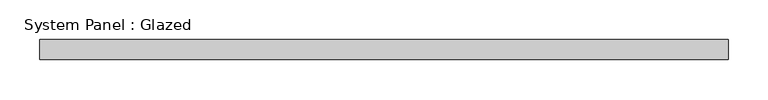
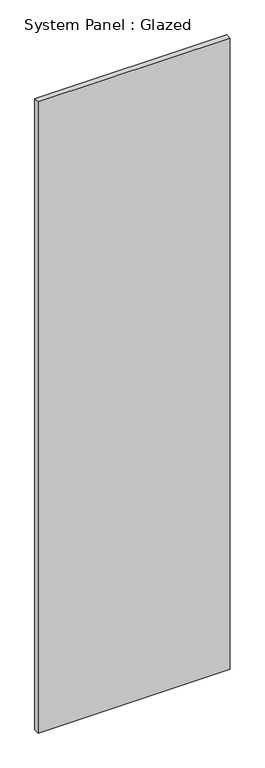
"""IFC4 building model written with IfcOpenShell, lengths in millimetres: plate geometry, System Panel : Glazed."""

from ifc_helpers import new_model, si_unit, origin, origin_with_axes, place, context, project, spatial, polyline, outline, extrude, source, transform, mapped, element, save


def system_panel_glazed_6dd91efc(model_context):
    return source(origin(), model_context, "Body", "SweptSolid", [
        extrude(outline(polyline([(431.8, 24.5), (-431.8, 24.5), (-431.8, 49.5), (431.8, 49.5), (431.8, 24.5)])), origin_with_axes(), (0.0, 0.0, 1.0), 3000.0),
    ])


if __name__ == "__main__":
    model = new_model("IFC4")
    model_context = context("Model", 3, world=origin())
    ifc_project = project(units=[si_unit("LENGTHUNIT", "METRE", prefix="MILLI")], contexts=[model_context])
    site = spatial("IfcSite", under=ifc_project)
    building = spatial("IfcBuilding", under=site)
    placement = place(None, origin())
    system_panel_glazed_shape = system_panel_glazed_6dd91efc(model_context)
    element("IfcPlate", 1, ObjectType="System Panel : Glazed", at=placement, inside=building, context=model_context, shape_type="MappedRepresentation", body=[
        mapped(system_panel_glazed_shape, transform((0.0, 0.0, 0.0), x_axis=(1.0, 0.0, 0.0), y_axis=(0.0, 1.0, 0.0), z_axis=(0.0, 0.0, 1.0))),
    ])
    save(model, "model.ifc")

# Revit data of these elements
# Type "System Panel : Glazed"
#   Keynote = "H11"
#   Construction Type Id = "GSP4R"
#   Analytic Construction = "1/8 in Pilkington single glazing"
#   Visual Light Transmittance = 0.9
#   Solar Heat Gain Coefficient = 0.86
#   Heat Transfer Coefficient (U) = 6.7069 W/(m²·K)
#   Define Thermal Properties by = 1
# Element 1 (IfcPlate, "System Panel : Glazed")
#   Materials on its faces: "Glass"
# Materials
#   "Glass": class "Glass", colour RGB 0 128 192, transparency 0.9, Description = "Soda Lime Glass", Cost = 0
